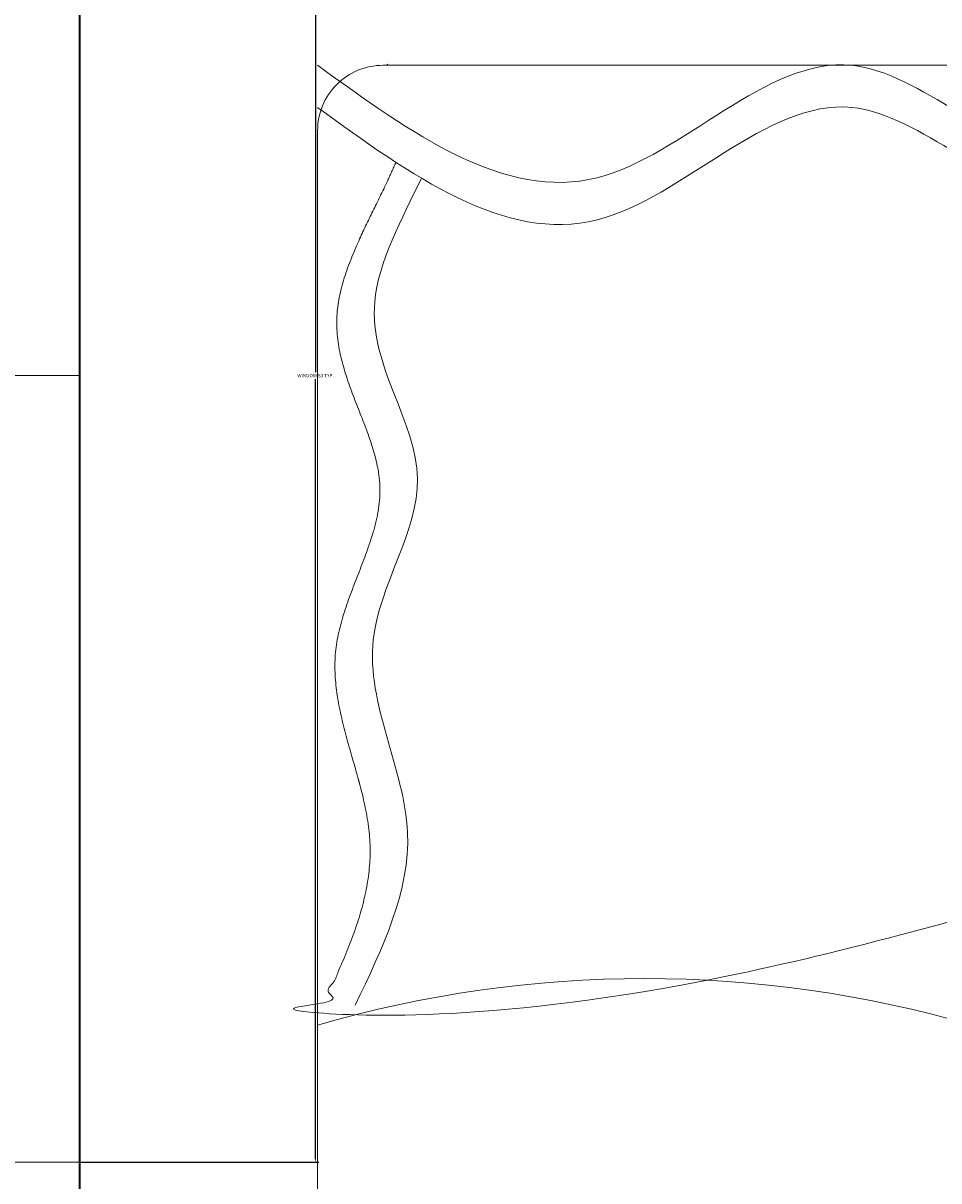
# Model space of a CAD drawing. Units: inches. Extents: x -61 to 1599, y -1316 to 257.
# Tile 120 of 204: x 85 to 133, y 27 to 88. Entities that reach past the tile are written whole.
import ezdxf

# ---------------------------------------------------------------- set-up
doc = ezdxf.new("R2010")
doc.units = ezdxf.units.IN
doc.header["$MEASUREMENT"] = 0
for name, color, linetype, lineweight in [('A-ANNO-DIMS', 2, 'Continuous', 18), ('FURNITURE', 83, 'Continuous', 18), ('WALLS', 4, 'Continuous', 35), ('WINDOWS', 220, 'Continuous', 18)]:
    doc.layers.add(name, color=color, linetype=linetype, lineweight=lineweight)
doc.styles.get("Standard").update_dxf_attribs({"font": 'arial.ttf'})
doc.dimstyles.get("Standard").update_dxf_attribs({"dimtxt": 0.18, "dimasz": 0.18, "dimexe": 0.18, "dimexo": 0.0625, "dimgap": 0.09, "dimtad": 0, "dimtih": 1, "dimtoh": 1, "dimdec": 0, "dimzin": 0, "dimdsep": 46, "dimlunit": 3, "dimtxsty": 'Standard', "dimcen": 0.09, "dimadec": 0, "dimazin": 0, "dimtfac": 1, "dimtdec": 0, "dimtofl": 0, "dimtmove": 0, "dimatfit": 3, "dimfxl": 1, "dimtolj": 1, "dimtzin": 0, "dimarcsym": 0})

# ---------------------------------------------------------------- blocks, each defined once
blk = doc.blocks.new('WIN-83IN')
blk.add_line((0, 0), (9, 0))
blk.add_lwpolyline([(9, 82.936), (4.5, 82.936), (4.5, 41.468), (9, 41.468)], close=True)
blk = doc.blocks.new('BED-DOUBLE')
blk.add_lwpolyline([(1.272, 88.537), (1.272, 3.449, 0.414214), (4.722, 0), (66.813, 0, 0.414214), (70.263, 3.449), (70.263, 88.537, 0.414214), (66.813, 91.987), (4.722, 91.987, 0.414214)], format="xyb", close=True)
blk.add_lwpolyline([(70.263, 41.387, -0.22309), (35.767, 41.387, 0.142156), (1.272, 41.387)], format="xyb")
for points, knots in [([(70.263, 91.987), (67.707, 89.379), (62.206, 83.764), (52.487, 96.724), (40.92, 82.741), (28.609, 96.737), (15.695, 81.527), (6.205, 88.409), (1.272, 91.987)], [0, 0, 0, 0, 9.176033, 19.753992, 33.150145, 45.209422, 59.881559, 75.764594, 75.764594, 75.764594, 75.764594]), ([(70.263, 89.765), (67.707, 87.157), (62.206, 81.542), (52.487, 94.502), (40.92, 80.519), (28.609, 94.515), (15.695, 79.305), (6.205, 86.187), (1.272, 89.765)], [0, 0, 0, 0, 9.176033, 19.753992, 33.150145, 45.209422, 59.881559, 75.764594, 75.764594, 75.764594, 75.764594]), ([(3.252, 42.437), (4.702, 45.448), (7.724, 51.72), (2.116, 61.25), (8.808, 70.52), (2.434, 77.934), (5.722, 83.908), (6.746, 86.037)], [0, 0, 0, 0, 8.27671, 17.241866, 24.903358, 33.244933, 38.427294, 38.427294, 38.427294, 38.427294])]:
    blk.add_open_spline(points, degree=3, knots=knots)
blk.add_open_spline([(5.011, 91.987), (4.986, 92.006), (4.961, 92.025), (4.936, 92.044)], degree=3)
blk.add_rational_spline([(70.263, 57.9), (59.862, 50.943), (48.595, 45.5), (36.681, 41.677), (36.463, 41.771), (36.247, 41.868), (36.032, 41.966), (24.597, 45.284), (12.692, 45.258), (1.272, 41.889), (2.723, 44.9), (5.745, 51.172), (0.137, 60.702), (6.828, 69.972), (0.109, 77.787), (4.354, 84.383), (5.398, 86.876)], [1, 0.993520320424, 0.993520320424, 1, 0.99997444972, 0.99997444972, 1, 0.973174868659, 0.973174868659, 1, 1, 1, 1, 1, 1, 1, 1], degree=3, knots=[0, 0, 0, 0, 0.279074, 0.279074, 0.279074, 0.296584, 0.296584, 0.296584, 0.865868, 0.865868, 0.865868, 9.142578, 18.107734, 25.769226, 34.110801, 40.441511, 40.441511, 40.441511, 40.441511])
blk = doc.blocks.new('*D644')
at = {"layer": 'A-ANNO-DIMS', "color": 0, "lineweight": -2, "transparency": 16777216}
for p, q in [((87.765, 111.301), (100.323, 111.301)), ((100.143, 111.121), (100.143, 70.016)), ((100.143, 28.545), (100.143, 69.65)), ((87.765, 28.365), (100.323, 28.365))]:
    blk.add_line(p, q, dxfattribs=at)
at = {"layer": 'A-ANNO-DIMS', "color": 0, "transparency": 16777216}
for points in [[(100.113, 111.121), (100.173, 111.121), (100.143, 111.301)], [(100.113, 28.545), (100.173, 28.545), (100.143, 28.365)]]:
    blk.add_solid(points, dxfattribs=at)
at = {"layer": 'DEFPOINTS', "color": 0, "transparency": 16777216}
for p in [(87.703, 111.301), (100.143, 111.301), (87.703, 28.365)]:
    blk.add_point(p, dxfattribs=at)
at = {"layer": 'A-ANNO-DIMS', "color": 0, "transparency": 16777216, "insert": (100.143, 69.833), "char_height": 0.18, "attachment_point": 5}
blk.add_mtext('\\A1;WINDOW 83 TYP.', dxfattribs=at)
blk = doc.blocks.new('*D645')
at = {"layer": 'A-ANNO-DIMS', "color": 0, "lineweight": -2, "transparency": 16777216}
for p, q in [((78.703, 28.303), (78.703, 15.745)), ((87.703, 28.303), (87.703, 15.745)), ((78.883, 15.925), (82.745, 15.925)), ((87.523, 15.925), (83.661, 15.925))]:
    blk.add_line(p, q, dxfattribs=at)
at = {"layer": 'A-ANNO-DIMS', "color": 0, "transparency": 16777216}
for points in [[(78.883, 15.955), (78.883, 15.895), (78.703, 15.925)], [(87.523, 15.955), (87.523, 15.895), (87.703, 15.925)]]:
    blk.add_solid(points, dxfattribs=at)
at = {"layer": 'DEFPOINTS', "color": 0, "transparency": 16777216}
for p in [(78.703, 28.365), (87.703, 28.365), (87.703, 15.925)]:
    blk.add_point(p, dxfattribs=at)
at = {"layer": 'A-ANNO-DIMS', "color": 0, "transparency": 16777216, "insert": (83.203, 15.925), "char_height": 0.18, "attachment_point": 5}
blk.add_mtext('\\A1;9 TYP.', dxfattribs=at)
blk = doc.blocks.new('*D687')
at = {"layer": 'A-ANNO-DIMS', "color": 0, "lineweight": -2, "transparency": 16777216}
for p, q in [((289.418, 181.677), (-61.077, 181.677)), ((-60.897, 181.497), (-60.897, -528.952)), ((-60.897, -1239.765), (-60.897, -529.316)), ((319.64, -1239.945), (-61.077, -1239.945))]:
    blk.add_line(p, q, dxfattribs=at)
at = {"layer": 'A-ANNO-DIMS', "color": 0, "transparency": 16777216}
for points in [[(-60.927, 181.497), (-60.867, 181.497), (-60.897, 181.677)], [(-60.927, -1239.765), (-60.867, -1239.765), (-60.897, -1239.945)]]:
    blk.add_solid(points, dxfattribs=at)
at = {"layer": 'DEFPOINTS', "color": 0, "transparency": 16777216}
for p in [(289.481, 181.677), (-60.897, -1239.945), (319.703, -1239.945)]:
    blk.add_point(p, dxfattribs=at)
at = {"layer": 'A-ANNO-DIMS', "color": 0, "transparency": 16777216, "insert": (-60.897, -529.134), "char_height": 0.18, "attachment_point": 5}
blk.add_mtext('\\A1;1421.6', dxfattribs=at)
blk = doc.blocks.new('*D700')
at = {"layer": 'A-ANNO-DIMS', "color": 0, "lineweight": -2, "transparency": 16777216}
for p, q in [((14.703, -616.882), (14.703, 257.457)), ((14.883, 257.277), (96.772, 257.277)), ((179.572, 257.277), (97.683, 257.277)), ((179.752, -616.882), (179.752, 257.457))]:
    blk.add_line(p, q, dxfattribs=at)
at = {"layer": 'A-ANNO-DIMS', "color": 0, "transparency": 16777216}
for points in [[(14.883, 257.307), (14.883, 257.247), (14.703, 257.277)], [(179.572, 257.307), (179.572, 257.247), (179.752, 257.277)]]:
    blk.add_solid(points, dxfattribs=at)
at = {"layer": 'DEFPOINTS', "color": 0, "transparency": 16777216}
for p in [(179.752, 257.277), (14.703, -616.945), (179.752, -616.945)]:
    blk.add_point(p, dxfattribs=at)
at = {"layer": 'A-ANNO-DIMS', "color": 0, "transparency": 16777216, "insert": (97.227, 257.277), "char_height": 0.18, "attachment_point": 5}
blk.add_mtext('\\A1;165.05', dxfattribs=at)

msp = doc.modelspace()

# ---------------------------------------------------------------- linework, layer by layer
at = {"layer": 'WALLS'}
msp.add_line((87.7028, 148.6771), (87.7028, -7.3229), dxfattribs=at)

# ---------------------------------------------------------------- block references
at = {"layer": 'FURNITURE'}
msp.add_blockref('BED-DOUBLE', (98.977, -5.797), dxfattribs=at)
at = {"layer": 'WINDOWS'}
msp.add_blockref('WIN-83IN', (78.703, 28.365), dxfattribs=at)

# ---------------------------------------------------------------- dimensions: what is measured, and where the dimension line sits
at = {"layer": 'A-ANNO-DIMS'}
dim = msp.add_linear_dim(base=(179.7521, 257.2771), p1=(14.7028, -616.9446), p2=(179.7521, -616.9446), dimstyle='Standard', override={"dimdec": 2, "dimlfac": 1, "dimrnd": 0, "dimzin": 0, "dimdsep": 46, "dimlunit": 2}, dxfattribs=at)
dim.commit()
dim.dimension.update_dxf_attribs({"geometry": '*D700', "text_midpoint": (97.2274, 257.2771)})
dim = msp.add_linear_dim(base=(-60.8972, -1239.9446), p1=(289.4807, 181.6771), p2=(319.7028, -1239.9446), angle=90, dimstyle='Standard', override={"dimdec": 1, "dimlfac": 1, "dimrnd": 0, "dimzin": 0, "dimdsep": 46, "dimlunit": 2}, dxfattribs=at)
dim.commit()
dim.dimension.update_dxf_attribs({"geometry": '*D687', "text_midpoint": (-60.8972, -529.1337)})
dim = msp.add_linear_dim(base=(100.1432, 111.3013), p1=(87.7028, 28.3651), p2=(87.7028, 111.3013), angle=90, text='WINDOW <> TYP.', dimstyle='Standard', override={"dimdec": 0, "dimlfac": 1, "dimrnd": 0, "dimzin": 0, "dimdsep": 46, "dimlunit": 2}, dxfattribs=at)
dim.commit()
dim.dimension.update_dxf_attribs({"geometry": '*D644', "text_midpoint": (100.1432, 69.8332)})
dim = msp.add_linear_dim(base=(87.7028, 15.9247), p1=(78.7028, 28.3651), p2=(87.7028, 28.3651), text='<> TYP.', dimstyle='Standard', override={"dimdec": 0, "dimlfac": 1, "dimrnd": 0, "dimzin": 0, "dimdsep": 46, "dimlunit": 2}, dxfattribs=at)
dim.commit()
dim.dimension.update_dxf_attribs({"geometry": '*D645', "text_midpoint": (83.2028, 15.9247)})

doc.saveas('drawing.dxf')
